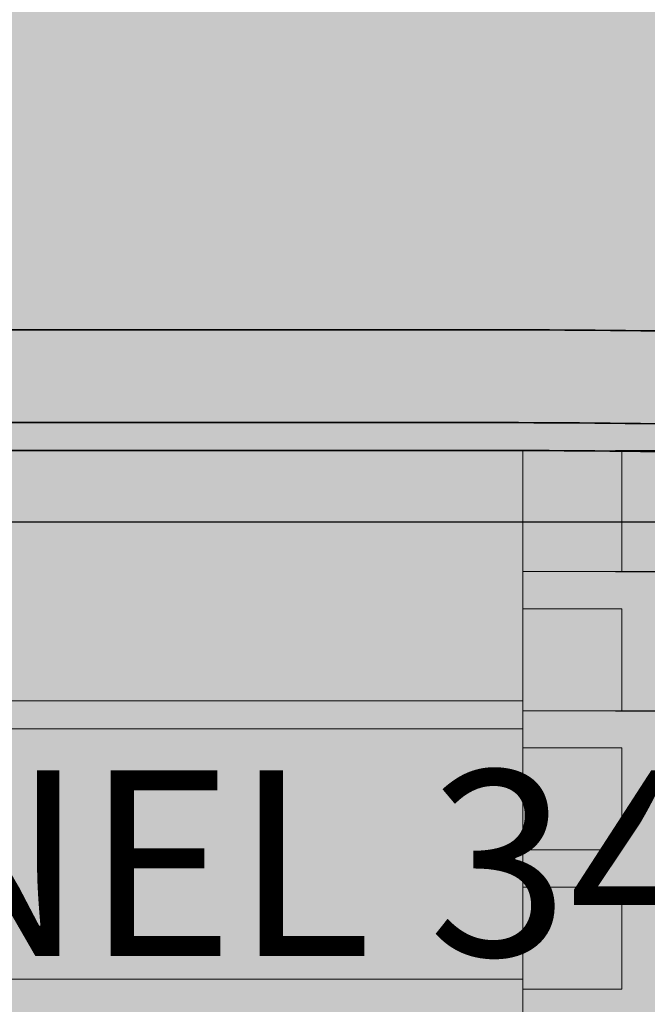
# Model space of a CAD drawing. Units: millimetres. Extents: x 130 to 1021, y 147 to 699.
# Tile 14 of 40: x 579 to 646, y 334 to 440. Entities that reach past the tile are written whole.
import ezdxf

# ---------------------------------------------------------------- set-up
doc = ezdxf.new("R2010")
doc.units = ezdxf.units.MM
doc.header["$MEASUREMENT"] = 0
for name, color, linetype, lineweight in [('A-ANNO-DIMS', 2, 'Continuous', 18), ('A-ELEV', 7, 'Continuous', 35), ('A-ELEV-PATT', 9, 'Continuous', 13), ('A-GLAZ', 4, 'Continuous', 18)]:
    doc.layers.add(name, color=color, linetype=linetype, lineweight=lineweight)
doc.styles.get("Standard").update_dxf_attribs({"font": 'arial.ttf'})
doc.dimstyles.get("Standard").update_dxf_attribs({"dimtxt": 20, "dimasz": 10, "dimexe": 10, "dimexo": 10, "dimgap": 5, "dimtad": 0, "dimtih": 1, "dimtoh": 1, "dimdec": 0, "dimzin": 0, "dimdsep": 46, "dimtxsty": 'Standard', "dimcen": 5, "dimadec": 0, "dimazin": 0, "dimtfac": 1, "dimtdec": 0, "dimtofl": 0, "dimtmove": 0, "dimatfit": 3, "dimfxl": 1, "dimtolj": 1, "dimtzin": 0, "dimarcsym": 0})

# ---------------------------------------------------------------- blocks, each defined once
blk = doc.blocks.new('*D7')
at = {"layer": 'A-ANNO-DIMS', "color": 0, "lineweight": -2, "transparency": 16777216}
for p, q in [((399.37, 349.45), (413.37, 349.45)), ((423.37, 349.45), (433.37, 349.45)), ((389.37, 344.55), (389.37, 339.45)), ((423.37, 344.55), (423.37, 339.45))]:
    blk.add_line(p, q, dxfattribs=at)
at = {"layer": 'A-ANNO-DIMS', "color": 0, "transparency": 16777216}
for points in [[(399.37, 351.11), (399.37, 347.78), (389.37, 349.45)], [(413.37, 351.11), (413.37, 347.78), (423.37, 349.45)]]:
    blk.add_solid(points, dxfattribs=at)
at = {"layer": 'Defpoints', "color": 0, "transparency": 16777216}
for p in [(389.37, 354.55), (423.37, 354.55), (423.37, 349.45)]:
    blk.add_point(p, dxfattribs=at)
at = {"layer": 'A-ANNO-DIMS', "color": 0, "transparency": 16777216, "insert": (582.04, 349.45), "char_height": 20, "attachment_point": 5}
blk.add_mtext('\\A1;DOOR PANEL 34 TYP.', dxfattribs=at)
blk = doc.blocks.new('*D11')
at = {"layer": 'A-ANNO-DIMS', "color": 0, "lineweight": -2, "transparency": 16777216}
for p, q in [((737.37, 648.7), (737.37, 149.74)), ((299.37, 566.95), (299.37, 149.74)), ((309.37, 159.74), (490.86, 159.74)), ((727.37, 159.74), (545.89, 159.74))]:
    blk.add_line(p, q, dxfattribs=at)
at = {"layer": 'A-ANNO-DIMS', "color": 0, "transparency": 16777216}
for points in [[(309.37, 161.41), (309.37, 158.07), (299.37, 159.74)], [(727.37, 161.41), (727.37, 158.07), (737.37, 159.74)]]:
    blk.add_solid(points, dxfattribs=at)
at = {"layer": 'Defpoints', "color": 0, "transparency": 16777216}
for p in [(737.37, 658.7), (299.37, 576.95), (737.37, 159.74)]:
    blk.add_point(p, dxfattribs=at)
at = {"layer": 'A-ANNO-DIMS', "color": 0, "transparency": 16777216, "insert": (518.37, 159.74), "char_height": 20, "attachment_point": 5}
blk.add_mtext('\\A1;438', dxfattribs=at)
blk = doc.blocks.new('*D24')
at = {"layer": 'A-ANNO-DIMS', "color": 0, "lineweight": -2, "transparency": 16777216}
for p, q in [((475.99, 209.04), (475.99, 696.25)), ((487.37, 671.95), (487.37, 696.25)), ((465.99, 686.25), (455.99, 686.25)), ((497.37, 686.25), (507.37, 686.25))]:
    blk.add_line(p, q, dxfattribs=at)
at = {"layer": 'A-ANNO-DIMS', "color": 0, "transparency": 16777216}
for points in [[(465.99, 687.91), (465.99, 684.58), (475.99, 686.25)], [(497.37, 687.91), (497.37, 684.58), (487.37, 686.25)]]:
    blk.add_solid(points, dxfattribs=at)
at = {"layer": 'Defpoints', "color": 0, "transparency": 16777216}
for p in [(487.37, 686.25), (487.37, 661.95), (475.99, 199.04)]:
    blk.add_point(p, dxfattribs=at)
at = {"layer": 'A-ANNO-DIMS', "color": 0, "transparency": 16777216, "insert": (553.02, 686.25), "char_height": 20, "attachment_point": 5}
blk.add_mtext('\\A1;11.385', dxfattribs=at)
blk = doc.blocks.new('*D27')
at = {"layer": 'A-ANNO-DIMS', "color": 0, "lineweight": -2, "transparency": 16777216}
for p, q in [((502.37, 593.95), (502.37, 696.25)), ((544.64, 396.26), (544.64, 696.25)), ((512.37, 686.25), (534.64, 686.25)), ((544.64, 686.25), (554.64, 686.25))]:
    blk.add_line(p, q, dxfattribs=at)
at = {"layer": 'A-ANNO-DIMS', "color": 0, "transparency": 16777216}
for points in [[(512.37, 687.91), (512.37, 684.58), (502.37, 686.25)], [(534.64, 687.91), (534.64, 684.58), (544.64, 686.25)]]:
    blk.add_solid(points, dxfattribs=at)
at = {"layer": 'Defpoints', "color": 0, "transparency": 16777216}
for p in [(544.64, 686.25), (502.37, 583.95), (544.64, 386.26)]:
    blk.add_point(p, dxfattribs=at)
at = {"layer": 'A-ANNO-DIMS', "color": 0, "transparency": 16777216, "insert": (593.78, 686.25), "char_height": 20, "attachment_point": 5}
blk.add_mtext('\\A1;42.26', dxfattribs=at)
blk = doc.blocks.new('*D28')
at = {"layer": 'A-ANNO-DIMS', "color": 0, "lineweight": -2, "transparency": 16777216}
for p, q in [((544.64, 396.26), (544.64, 696.25)), ((552.37, 593.95), (552.37, 696.25)), ((534.64, 686.25), (524.64, 686.25)), ((562.37, 686.25), (572.37, 686.25))]:
    blk.add_line(p, q, dxfattribs=at)
at = {"layer": 'A-ANNO-DIMS', "color": 0, "transparency": 16777216}
for points in [[(534.64, 687.91), (534.64, 684.58), (544.64, 686.25)], [(562.37, 687.91), (562.37, 684.58), (552.37, 686.25)]]:
    blk.add_solid(points, dxfattribs=at)
at = {"layer": 'Defpoints', "color": 0, "transparency": 16777216}
for p in [(552.37, 686.25), (552.37, 583.95), (544.64, 386.26)]:
    blk.add_point(p, dxfattribs=at)
at = {"layer": 'A-ANNO-DIMS', "color": 0, "transparency": 16777216, "insert": (611.06, 686.25), "char_height": 20, "attachment_point": 5}
blk.add_mtext('\\A1;7.738', dxfattribs=at)
blk = doc.blocks.new('*D51')
at = {"layer": 'A-ANNO-DIMS', "color": 0, "lineweight": -2, "transparency": 16777216}
for p, q in [((554.64, 386.26), (771.67, 386.26)), ((761.67, 376.26), (761.67, 348.67)), ((761.67, 290.66), (761.67, 318.25)), ((554.64, 280.66), (771.67, 280.66))]:
    blk.add_line(p, q, dxfattribs=at)
at = {"layer": 'A-ANNO-DIMS', "color": 0, "transparency": 16777216}
for points in [[(760.01, 376.26), (763.34, 376.26), (761.67, 386.26)], [(760.01, 290.66), (763.34, 290.66), (761.67, 280.66)]]:
    blk.add_solid(points, dxfattribs=at)
at = {"layer": 'Defpoints', "color": 0, "transparency": 16777216}
for p in [(544.64, 386.26), (761.67, 386.26), (544.64, 280.66)]:
    blk.add_point(p, dxfattribs=at)
at = {"layer": 'A-ANNO-DIMS', "color": 0, "transparency": 16777216, "insert": (761.67, 333.46), "char_height": 20, "attachment_point": 5}
blk.add_mtext('\\A1;105.6', dxfattribs=at)
blk = doc.blocks.new('*D52')
at = {"layer": 'A-ANNO-DIMS', "color": 0, "lineweight": -2, "transparency": 16777216}
for p, q in [((761.67, 403.95), (761.67, 413.95)), ((761.67, 413.95), (771.67, 413.95)), ((642.82, 393.95), (771.67, 393.95)), ((554.64, 386.26), (771.67, 386.26)), ((761.67, 376.26), (761.67, 366.26))]:
    blk.add_line(p, q, dxfattribs=at)
at = {"layer": 'A-ANNO-DIMS', "color": 0, "transparency": 16777216}
for points in [[(760.01, 403.95), (763.34, 403.95), (761.67, 393.95)], [(760.01, 376.26), (763.34, 376.26), (761.67, 386.26)]]:
    blk.add_solid(points, dxfattribs=at)
at = {"layer": 'Defpoints', "color": 0, "transparency": 16777216}
for p in [(632.82, 393.95), (761.67, 393.95), (544.64, 386.26)]:
    blk.add_point(p, dxfattribs=at)
at = {"layer": 'A-ANNO-DIMS', "color": 0, "transparency": 16777216, "insert": (810.34, 413.95), "char_height": 20, "attachment_point": 5}
blk.add_mtext('\\A1;7.683', dxfattribs=at)
blk = doc.blocks.new('*D53')
at = {"layer": 'A-ANNO-DIMS', "color": 0, "lineweight": -2, "transparency": 16777216}
for p, q in [((761.67, 413.69), (761.67, 423.69)), ((761.67, 423.69), (771.67, 423.69)), ((747.37, 403.69), (771.67, 403.69)), ((642.82, 393.95), (771.67, 393.95)), ((761.67, 383.95), (761.67, 373.95))]:
    blk.add_line(p, q, dxfattribs=at)
at = {"layer": 'A-ANNO-DIMS', "color": 0, "transparency": 16777216}
for points in [[(760.01, 413.69), (763.34, 413.69), (761.67, 403.69)], [(760.01, 383.95), (763.34, 383.95), (761.67, 393.95)]]:
    blk.add_solid(points, dxfattribs=at)
at = {"layer": 'Defpoints', "color": 0, "transparency": 16777216}
for p in [(737.37, 403.69), (761.67, 403.69), (632.82, 393.95)]:
    blk.add_point(p, dxfattribs=at)
at = {"layer": 'A-ANNO-DIMS', "color": 0, "transparency": 16777216, "insert": (810.42, 423.69), "char_height": 20, "attachment_point": 5}
blk.add_mtext('\\A1;9.743', dxfattribs=at)
blk = doc.blocks.new('*D54')
at = {"layer": 'A-ANNO-DIMS', "color": 0, "lineweight": -2, "transparency": 16777216}
for p, q in [((761.67, 473.95), (761.67, 483.95)), ((497.37, 463.95), (771.67, 463.95)), ((747.37, 403.69), (771.67, 403.69)), ((761.67, 393.69), (761.67, 383.69))]:
    blk.add_line(p, q, dxfattribs=at)
at = {"layer": 'A-ANNO-DIMS', "color": 0, "transparency": 16777216}
for points in [[(760.01, 473.95), (763.34, 473.95), (761.67, 463.95)], [(760.01, 393.69), (763.34, 393.69), (761.67, 403.69)]]:
    blk.add_solid(points, dxfattribs=at)
at = {"layer": 'Defpoints', "color": 0, "transparency": 16777216}
for p in [(487.37, 463.95), (761.67, 463.95), (737.37, 403.69)]:
    blk.add_point(p, dxfattribs=at)
at = {"layer": 'A-ANNO-DIMS', "color": 0, "transparency": 16777216, "insert": (761.67, 433.82), "char_height": 20, "attachment_point": 5}
blk.add_mtext('\\A1;60.26', dxfattribs=at)
blk = doc.blocks.new('*D61')
at = {"layer": 'A-ANNO-DIMS', "color": 0, "lineweight": -2, "transparency": 16777216}
for p, q in [((761.67, 390.89), (761.67, 400.89)), ((642.82, 380.89), (771.67, 380.89)), ((642.82, 365.89), (771.67, 365.89)), ((761.67, 355.89), (761.67, 345.89)), ((761.67, 345.89), (751.67, 345.89))]:
    blk.add_line(p, q, dxfattribs=at)
at = {"layer": 'A-ANNO-DIMS', "color": 0, "transparency": 16777216}
for points in [[(760.01, 390.89), (763.34, 390.89), (761.67, 380.89)], [(760.01, 355.89), (763.34, 355.89), (761.67, 365.89)]]:
    blk.add_solid(points, dxfattribs=at)
at = {"layer": 'Defpoints', "color": 0, "transparency": 16777216}
for p in [(632.82, 380.89), (632.82, 365.89), (761.67, 365.89)]:
    blk.add_point(p, dxfattribs=at)
at = {"layer": 'A-ANNO-DIMS', "color": 0, "transparency": 16777216, "insert": (733.22, 345.89), "char_height": 20, "attachment_point": 5}
blk.add_mtext('\\A1;15', dxfattribs=at)
blk = doc.blocks.new('*D65')
at = {"layer": 'A-ANNO-DIMS', "color": 0, "lineweight": -2, "transparency": 16777216}
for p, q in [((495.46, 509.13), (472.51, 423.11)), ((505.46, 509.13), (495.46, 509.13)), ((427.37, 248.98), (427.37, 258.98)), ((422.37, 253.98), (432.37, 253.98))]:
    blk.add_line(p, q, dxfattribs=at)
at = {"layer": 'A-ANNO-DIMS', "color": 0, "transparency": 16777216}
blk.add_solid([(470.9, 423.54), (474.12, 422.68), (469.93, 413.45)], dxfattribs=at)
at = {"layer": 'Defpoints', "color": 0, "transparency": 16777216}
for p in [(469.93, 413.45), (427.37, 253.98)]:
    blk.add_point(p, dxfattribs=at)
at = {"layer": 'A-ANNO-DIMS', "color": 0, "transparency": 16777216, "insert": (561.62, 509.13), "char_height": 20, "attachment_point": 5}
blk.add_mtext('\\A1;R165.05', dxfattribs=at)
blk = doc.blocks.new('*D67')
at = {"layer": 'A-ANNO-DIMS', "color": 0, "lineweight": -2, "transparency": 16777216}
for p, q in [((479.76, 492.43), (462.14, 412.22)), ((489.76, 492.43), (479.76, 492.43)), ((427.07, 247.5), (427.07, 257.5)), ((422.07, 252.5), (432.07, 252.5))]:
    blk.add_line(p, q, dxfattribs=at)
at = {"layer": 'A-ANNO-DIMS', "color": 0, "transparency": 16777216}
blk.add_solid([(460.52, 412.58), (463.77, 411.87), (460, 402.46)], dxfattribs=at)
at = {"layer": 'Defpoints', "color": 0, "transparency": 16777216}
for p in [(460, 402.46), (427.07, 252.5)]:
    blk.add_point(p, dxfattribs=at)
at = {"layer": 'A-ANNO-DIMS', "color": 0, "transparency": 16777216, "insert": (545.84, 492.43), "char_height": 20, "attachment_point": 5}
blk.add_mtext('\\A1;R153.53', dxfattribs=at)
blk = doc.blocks.new('*D69')
at = {"layer": 'A-ANNO-DIMS', "color": 0, "lineweight": -2, "transparency": 16777216}
for p, q in [((507.75, 572.26), (483.09, 501.81)), ((517.75, 572.26), (507.75, 572.26)), ((433.19, 354.23), (433.19, 364.23)), ((428.19, 359.23), (438.19, 359.23))]:
    blk.add_line(p, q, dxfattribs=at)
at = {"layer": 'A-ANNO-DIMS', "color": 0, "transparency": 16777216}
blk.add_solid([(481.52, 502.36), (484.66, 501.26), (479.79, 492.37)], dxfattribs=at)
at = {"layer": 'Defpoints', "color": 0, "transparency": 16777216}
for p in [(479.79, 492.37), (433.19, 359.23)]:
    blk.add_point(p, dxfattribs=at)
at = {"layer": 'A-ANNO-DIMS', "color": 0, "transparency": 16777216, "insert": (573.82, 572.26), "char_height": 20, "attachment_point": 5}
blk.add_mtext('\\A1;R141.06', dxfattribs=at)
blk = doc.blocks.new('*D71')
at = {"layer": 'A-ANNO-DIMS', "color": 0, "lineweight": -2, "transparency": 16777216}
for p, q in [((492.11, 581.61), (472.54, 512.67)), ((502.11, 581.61), (492.11, 581.61)), ((432.65, 367.11), (432.65, 377.11)), ((427.65, 372.11), (437.65, 372.11))]:
    blk.add_line(p, q, dxfattribs=at)
at = {"layer": 'A-ANNO-DIMS', "color": 0, "transparency": 16777216}
blk.add_solid([(470.94, 513.12), (474.15, 512.21), (469.81, 503.05)], dxfattribs=at)
at = {"layer": 'Defpoints', "color": 0, "transparency": 16777216}
for p in [(469.81, 503.05), (432.65, 372.11)]:
    blk.add_point(p, dxfattribs=at)
at = {"layer": 'A-ANNO-DIMS', "color": 0, "transparency": 16777216, "insert": (548.49, 581.61), "char_height": 20, "attachment_point": 5}
blk.add_mtext('\\A1;R136.1', dxfattribs=at)

msp = doc.modelspace()

# ---------------------------------------------------------------- hatches: boundary and pattern name
at = {"layer": 'A-ELEV-PATT'}
h = msp.add_hatch(color=256, dxfattribs=at)
h.dxf.hatch_style = 1
h.paths.add_polyline_path([(737.3738, 658.6988, 0.01359606), (632.4019, 661.9473), (607.3738, 661.9473), (487.3738, 661.9473), (487.3738, 649.9473), (607.3738, 649.9473), (632.3794, 649.9473, -0.01368411), (737.3738, 646.6784)])
h.paths.add_polyline_path([(732.3738, 643.9599, 0.01305286), (632.3738, 646.9473), (607.3738, 646.9473), (487.3738, 646.9473), (487.3738, 596.9473), (632.3738, 596.9473, -0.01305286), (732.3738, 593.9599)])
h.paths.add_polyline_path([(737.3738, 593.6732, 0.01370629), (632.3738, 596.9473), (487.3738, 596.9473), (487.3738, 586.9473), (632.355, 586.9473, -0.01378075), (737.3738, 583.6559)])
h.paths.add_polyline_path([(447.3738, 646.9473), (307.3738, 646.9473), (302.3738, 646.9473), (302.3738, 634.9473), (447.3738, 634.9473)])
h.paths.add_polyline_path([(447.3738, 631.9473), (307.3738, 631.9473), (307.3738, 586.9473), (447.3738, 586.9473)])
h.paths.add_polyline_path([(447.3738, 586.9473), (307.3738, 586.9473), (302.3738, 586.9473), (302.3738, 576.9473), (447.3738, 576.9473)])
h.paths.add_polyline_path([(447.3738, 573.9473), (367.3738, 573.9473), (367.3738, 539.9473), (447.3738, 539.9473)])
h.paths.add_polyline_path([(447.3738, 537.9473), (367.3738, 537.9473), (367.3738, 507.9473), (400.392, 507.4253, -0.00172798), (401.3281, 507.6451, -0.52200255), (425.6117, 511.0391, -0.03918489), (447.3738, 510.4359), (447.3738, 510.7883)])
h.paths.add_polyline_path([(394.7238, 505.9473), (367.3738, 505.9473), (367.3738, 476.9473, -0.0146512), (375.8501, 480.2159), (376.1506, 499.2266, -0.03554194)])
h.paths.add_polyline_path([(632.3738, 583.9473), (552.3738, 583.9473), (552.3738, 550.9473), (632.3738, 550.9473)])
h.paths.add_polyline_path([(632.3738, 548.9473), (552.3738, 548.9473), (552.3738, 515.9473), (632.3738, 515.9473)])
h.paths.add_polyline_path([(632.3738, 513.9473), (552.3738, 513.9473), (552.3738, 476.9473), (632.3738, 476.9473)])
h.paths.add_polyline_path([(737.3738, 473.6903, 0.01363261), (632.3926, 476.9473), (552.3738, 476.9473), (487.3738, 476.9473), (487.3738, 466.9473), (632.3738, 466.9473, -0.01370629), (737.3738, 463.6732)])
h.paths.add_polyline_path([(732.3738, 460.9552, 0.01307409), (632.3681, 463.9473), (487.3738, 463.9473), (487.3738, 407.735, -0.00322862), (489.3544, 406.9473), (632.3926, 406.9473, -0.01298259), (732.3738, 403.9755)])
h.paths.add_polyline_path([(487.3738, 463.9473, 0.20132998), (367.3738, 463.9473), (367.3738, 407.735, -0.18820307), (487.3738, 407.735)])
h.paths.add_polyline_path([(367.3738, 476.9473), (367.3738, 466.9473, -0.20133085), (487.3738, 466.9473), (487.3738, 476.9473, 0.20132998)])
h.paths.add_polyline_path([(367.3738, 463.9473), (307.3738, 463.9473), (307.3738, 401.9473), (357.9413, 401.9473), (367.3738, 407.735)])
h.paths.add_polyline_path([(367.3738, 476.9473), (302.3738, 476.9473), (302.3738, 466.9473), (367.3738, 466.9473)])
h.paths.add_polyline_path([(632.8184, 366.9453), (552.3738, 366.9453), (552.3738, 393.9473), (632.8184, 393.9473)])
h.paths.add_polyline_path([(632.8184, 357.2114), (632.8184, 363.9453), (552.3738, 363.9453), (552.3738, 357.2114), (552.3738, 336.9453), (632.8184, 336.9453)])
h.paths.add_polyline_path([(632.8184, 333.9453), (552.3738, 333.9453), (552.3738, 306.9453), (632.8184, 306.9453)])
h.paths.add_polyline_path([(632.8184, 303.9453), (552.3738, 303.9453), (552.3738, 273.9473), (632.355, 273.9473, 0.00006077), (632.8184, 273.9491)])
h.paths.add_polyline_path([(737.3738, 403.6903, 0.01363261), (632.3926, 406.9473), (489.3544, 406.9473, 0.19154808), (367.3738, 407.735), (367.3738, 396.9473, -0.20133085), (487.3738, 396.9473), (632.3738, 396.9473, -0.01370629), (737.3738, 393.6732)])
h.paths.add_polyline_path([(357.9413, 401.9473), (307.3738, 401.9473), (307.3738, 391.9473), (357.9413, 391.9473)])
h.paths.add_polyline_path([(357.9413, 357.2114), (357.9413, 388.9473), (307.3738, 388.9473), (307.3738, 357.2114), (307.3738, 273.9473), (357.9413, 273.9473)])
h.paths.add_polyline_path([(732.3738, 263.93, -0.0130317), (632.3794, 260.9473), (466.7667, 260.9473), (466.7667, 240.9473), (469.8406, 236.978), (469.8406, 221.978), (472.9145, 218.0087), (472.9145, 213.9473), (607.3738, 213.9473), (732.3738, 213.9473)])
h.paths.add_polyline_path([(732.3738, 290.889), (722.479, 290.889), (722.479, 301.889), (732.3738, 301.889), (732.3738, 305.889), (722.479, 305.889), (722.479, 316.889), (732.3738, 316.889), (732.3738, 320.889), (722.479, 320.889), (722.479, 331.889), (732.3738, 331.889), (732.3738, 335.889), (722.479, 335.889), (722.479, 346.889), (732.3738, 346.889), (732.3738, 350.889), (722.479, 350.889), (722.479, 361.889), (732.3738, 361.889), (732.3738, 365.889), (722.479, 365.889), (722.479, 376.889), (732.3738, 376.889), (732.3738, 380.889), (722.479, 380.889), (722.479, 391.4848, 0.00052326), (718.479, 391.6843), (718.479, 380.889), (707.479, 380.889), (707.479, 392.1896, 0.00052307), (703.479, 392.3576), (703.479, 380.889), (692.479, 380.889), (692.479, 392.7765, 0.00052292), (688.479, 392.9131), (688.479, 380.889), (677.479, 380.889), (677.479, 393.2456, 0.00052279), (673.479, 393.3508), (673.479, 380.889), (662.479, 380.889), (662.479, 393.597, 0.0005227), (658.479, 393.6709), (658.479, 380.889), (647.479, 380.889), (647.479, 393.8308, 0.00052264), (643.479, 393.8732), (643.479, 380.889), (632.8184, 380.889), (632.8184, 376.889), (643.479, 376.889), (643.479, 365.889), (632.8184, 365.889), (632.8184, 361.889), (643.479, 361.889), (643.479, 350.889), (632.8184, 350.889), (632.8184, 346.889), (643.479, 346.889), (643.479, 335.889), (632.8184, 335.889), (632.8184, 331.889), (643.479, 331.889), (643.479, 320.889), (632.8184, 320.889), (632.8184, 316.889), (643.479, 316.889), (643.479, 305.889), (632.8184, 305.889), (632.8184, 301.889), (643.479, 301.889), (643.479, 290.889), (632.8184, 290.889), (632.8184, 286.889), (643.479, 286.889), (643.479, 274.0217, 0.00052456), (647.479, 274.0643), (647.479, 286.889), (658.479, 286.889), (658.479, 274.2248, 0.00052462), (662.479, 274.2989), (662.479, 286.889), (673.479, 286.889), (673.479, 274.546, 0.00052471), (677.479, 274.6516), (677.479, 286.889), (688.479, 286.889), (688.479, 274.9853, 0.00052484), (692.479, 275.1224), (692.479, 286.889), (703.479, 286.889), (703.479, 275.5429, 0.000525), (707.479, 275.7115), (707.479, 286.889), (718.479, 286.889), (718.479, 276.2187, 0.00052519), (722.479, 276.4189), (722.479, 286.889), (732.3738, 286.889)])
h.paths.add_polyline_path([(718.479, 290.889), (707.479, 290.889), (707.479, 301.889), (718.479, 301.889)], flags=16)
h.paths.add_polyline_path([(703.479, 290.889), (692.479, 290.889), (692.479, 301.889), (703.479, 301.889)], flags=16)
h.paths.add_polyline_path([(718.479, 305.889), (707.479, 305.889), (707.479, 316.889), (718.479, 316.889)], flags=16)
h.paths.add_polyline_path([(703.479, 305.889), (692.479, 305.889), (692.479, 316.889), (703.479, 316.889)], flags=16)
h.paths.add_polyline_path([(688.479, 290.889), (677.479, 290.889), (677.479, 301.889), (688.479, 301.889)], flags=16)
h.paths.add_polyline_path([(718.479, 320.889), (707.479, 320.889), (707.479, 331.889), (718.479, 331.889)], flags=16)
h.paths.add_polyline_path([(688.479, 305.889), (677.479, 305.889), (677.479, 316.889), (688.479, 316.889)], flags=16)
h.paths.add_polyline_path([(703.479, 320.889), (692.479, 320.889), (692.479, 331.889), (703.479, 331.889)], flags=16)
h.paths.add_polyline_path([(688.479, 320.889), (677.479, 320.889), (677.479, 331.889), (688.479, 331.889)], flags=16)
h.paths.add_polyline_path([(673.479, 290.889), (662.479, 290.889), (662.479, 301.889), (673.479, 301.889)], flags=16)
h.paths.add_polyline_path([(718.479, 335.889), (707.479, 335.889), (707.479, 346.889), (718.479, 346.889)], flags=16)
h.paths.add_polyline_path([(673.479, 305.889), (662.479, 305.889), (662.479, 316.889), (673.479, 316.889)], flags=16)
h.paths.add_polyline_path([(703.479, 335.889), (692.479, 335.889), (692.479, 346.889), (703.479, 346.889)], flags=16)
h.paths.add_polyline_path([(673.479, 320.889), (662.479, 320.889), (662.479, 331.889), (673.479, 331.889)], flags=16)
h.paths.add_polyline_path([(688.479, 335.889), (677.479, 335.889), (677.479, 346.889), (688.479, 346.889)], flags=16)
h.paths.add_polyline_path([(658.479, 290.889), (647.479, 290.889), (647.479, 301.889), (658.479, 301.889)], flags=16)
h.paths.add_polyline_path([(718.479, 350.889), (707.479, 350.889), (707.479, 361.889), (718.479, 361.889)], flags=16)
h.paths.add_polyline_path([(658.479, 305.889), (647.479, 305.889), (647.479, 316.889), (658.479, 316.889)], flags=16)
h.paths.add_polyline_path([(703.479, 350.889), (692.479, 350.889), (692.479, 361.889), (703.479, 361.889)], flags=16)
h.paths.add_polyline_path([(673.479, 335.889), (662.479, 335.889), (662.479, 346.889), (673.479, 346.889)], flags=16)
h.paths.add_polyline_path([(658.479, 320.889), (647.479, 320.889), (647.479, 331.889), (658.479, 331.889)], flags=16)
h.paths.add_polyline_path([(688.479, 350.889), (677.479, 350.889), (677.479, 361.889), (688.479, 361.889)], flags=16)
h.paths.add_polyline_path([(718.479, 365.889), (707.479, 365.889), (707.479, 376.889), (718.479, 376.889)], flags=16)
h.paths.add_polyline_path([(658.479, 335.889), (647.479, 335.889), (647.479, 346.889), (658.479, 346.889)], flags=16)
h.paths.add_polyline_path([(673.479, 350.889), (662.479, 350.889), (662.479, 361.889), (673.479, 361.889)], flags=16)
h.paths.add_polyline_path([(703.479, 365.889), (692.479, 365.889), (692.479, 376.889), (703.479, 376.889)], flags=16)
h.paths.add_polyline_path([(688.479, 365.889), (677.479, 365.889), (677.479, 376.889), (688.479, 376.889)], flags=16)
h.paths.add_polyline_path([(658.479, 350.889), (647.479, 350.889), (647.479, 361.889), (658.479, 361.889)], flags=16)
h.paths.add_polyline_path([(673.479, 365.889), (662.479, 365.889), (662.479, 376.889), (673.479, 376.889)], flags=16)
h.paths.add_polyline_path([(658.479, 365.889), (647.479, 365.889), (647.479, 376.889), (658.479, 376.889)], flags=16)
h.paths.add_polyline_path([(732.3738, 503.9786), (722.3392, 503.9786), (722.3392, 514.9786), (732.3738, 514.9786), (732.3738, 518.9786), (722.3392, 518.9786), (722.3392, 529.9786), (732.3738, 529.9786), (732.3738, 533.9786), (722.3392, 533.9786), (722.3392, 544.9786), (732.3738, 544.9786), (732.3738, 546.9473), (732.3738, 548.9786), (722.3392, 548.9786), (722.3392, 559.9786), (732.3738, 559.9786), (732.3738, 563.9786), (722.3392, 563.9786), (722.3392, 574.9786), (732.3738, 574.9786), (732.3738, 578.9786), (722.3392, 578.9786), (722.3392, 581.4789, 0.00052601), (718.3392, 581.6791), (718.3392, 578.9786), (707.3392, 578.9786), (707.3392, 582.1863, 0.00052582), (703.3392, 582.355), (703.3392, 578.9786), (692.3392, 578.9786), (692.3392, 582.7752, 0.00052566), (688.3392, 582.9123), (688.3392, 578.9786), (677.3392, 578.9786), (677.3392, 583.2457, 0.00052554), (673.3392, 583.3512), (673.3392, 578.9786), (662.3392, 578.9786), (662.3392, 583.5978, 0.00052545), (658.3392, 583.6718), (658.3392, 578.9786), (647.3392, 578.9786), (647.3392, 583.8317, 0.00052539), (643.3392, 583.8741), (643.3392, 578.9786), (632.3738, 578.9786), (632.3738, 574.9786), (643.3392, 574.9786), (643.3392, 563.9786), (632.3738, 563.9786), (632.3738, 559.9786), (643.3392, 559.9786), (643.3392, 548.9786), (632.3738, 548.9786), (632.3738, 544.9786), (643.3392, 544.9786), (643.3392, 533.9786), (632.3738, 533.9786), (632.3738, 529.9786), (643.3392, 529.9786), (643.3392, 518.9786), (632.3738, 518.9786), (632.3738, 515.9473), (632.3738, 514.9786), (643.3392, 514.9786), (643.3392, 503.9786), (632.3738, 503.9786), (632.3738, 499.9786), (643.3392, 499.9786), (643.3392, 488.9786), (632.3738, 488.9786), (632.3738, 484.9786), (643.3392, 484.9786), (643.3392, 476.8751, -0.00051911), (647.3392, 476.8332), (647.3392, 484.9786), (658.3392, 484.9786), (658.3392, 476.6752, -0.00051917), (662.3392, 476.6022), (662.3392, 484.9786), (673.3392, 484.9786), (673.3392, 476.3585, -0.00051926), (677.3392, 476.2543), (677.3392, 484.9786), (688.3392, 484.9786), (688.3392, 475.9248, -0.00051938), (692.3392, 475.7894), (692.3392, 484.9786), (703.3392, 484.9786), (703.3392, 475.3741, -0.00051953), (707.3392, 475.2075), (707.3392, 484.9786), (718.3392, 484.9786), (718.3392, 474.7064, -0.00051972), (722.3392, 474.5086), (722.3392, 484.9786), (732.3738, 484.9786), (732.3738, 488.9786), (722.3392, 488.9786), (722.3392, 499.9786), (732.3738, 499.9786)])
h.paths.add_polyline_path([(718.3392, 503.9786), (707.3392, 503.9786), (707.3392, 514.9786), (718.3392, 514.9786)], flags=16)
h.paths.add_polyline_path([(718.3392, 499.9786), (718.3392, 488.9786), (707.3392, 488.9786), (707.3392, 499.9786)], flags=16)
h.paths.add_polyline_path([(718.3392, 518.9786), (707.3392, 518.9786), (707.3392, 529.9786), (718.3392, 529.9786)], flags=16)
h.paths.add_polyline_path([(703.3392, 503.9786), (692.3392, 503.9786), (692.3392, 514.9786), (703.3392, 514.9786)], flags=16)
h.paths.add_polyline_path([(703.3392, 499.9786), (703.3392, 488.9786), (692.3392, 488.9786), (692.3392, 499.9786)], flags=16)
h.paths.add_polyline_path([(703.3392, 518.9786), (692.3392, 518.9786), (692.3392, 529.9786), (703.3392, 529.9786)], flags=16)
h.paths.add_polyline_path([(718.3392, 533.9786), (707.3392, 533.9786), (707.3392, 544.9786), (718.3392, 544.9786)], flags=16)
h.paths.add_polyline_path([(688.3392, 503.9786), (677.3392, 503.9786), (677.3392, 514.9786), (688.3392, 514.9786)], flags=16)
h.paths.add_polyline_path([(688.3392, 499.9786), (688.3392, 488.9786), (677.3392, 488.9786), (677.3392, 499.9786)], flags=16)
h.paths.add_polyline_path([(703.3392, 533.9786), (692.3392, 533.9786), (692.3392, 544.9786), (703.3392, 544.9786)], flags=16)
h.paths.add_polyline_path([(688.3392, 518.9786), (677.3392, 518.9786), (677.3392, 529.9786), (688.3392, 529.9786)], flags=16)
h.paths.add_polyline_path([(688.3392, 533.9786), (677.3392, 533.9786), (677.3392, 544.9786), (688.3392, 544.9786)], flags=16)
h.paths.add_polyline_path([(718.3392, 548.9786), (707.3392, 548.9786), (707.3392, 559.9786), (718.3392, 559.9786)], flags=16)
h.paths.add_polyline_path([(673.3392, 503.9786), (662.3392, 503.9786), (662.3392, 514.9786), (673.3392, 514.9786)], flags=16)
h.paths.add_polyline_path([(673.3392, 499.9786), (673.3392, 488.9786), (662.3392, 488.9786), (662.3392, 499.9786)], flags=16)
h.paths.add_polyline_path([(703.3392, 548.9786), (692.3392, 548.9786), (692.3392, 559.9786), (703.3392, 559.9786)], flags=16)
h.paths.add_polyline_path([(673.3392, 518.9786), (662.3392, 518.9786), (662.3392, 529.9786), (673.3392, 529.9786)], flags=16)
h.paths.add_polyline_path([(688.3392, 548.9786), (677.3392, 548.9786), (677.3392, 559.9786), (688.3392, 559.9786)], flags=16)
h.paths.add_polyline_path([(673.3392, 533.9786), (662.3392, 533.9786), (662.3392, 544.9786), (673.3392, 544.9786)], flags=16)
h.paths.add_polyline_path([(718.3392, 563.9786), (707.3392, 563.9786), (707.3392, 574.9786), (718.3392, 574.9786)], flags=16)
h.paths.add_polyline_path([(658.3392, 503.9786), (647.3392, 503.9786), (647.3392, 514.9786), (658.3392, 514.9786)], flags=16)
h.paths.add_polyline_path([(658.3392, 499.9786), (658.3392, 488.9786), (647.3392, 488.9786), (647.3392, 499.9786)], flags=16)
h.paths.add_polyline_path([(703.3392, 563.9786), (692.3392, 563.9786), (692.3392, 574.9786), (703.3392, 574.9786)], flags=16)
h.paths.add_polyline_path([(658.3392, 518.9786), (647.3392, 518.9786), (647.3392, 529.9786), (658.3392, 529.9786)], flags=16)
h.paths.add_polyline_path([(673.3392, 548.9786), (662.3392, 548.9786), (662.3392, 559.9786), (673.3392, 559.9786)], flags=16)
h.paths.add_polyline_path([(688.3392, 563.9786), (677.3392, 563.9786), (677.3392, 574.9786), (688.3392, 574.9786)], flags=16)
h.paths.add_polyline_path([(658.3392, 533.9786), (647.3392, 533.9786), (647.3392, 544.9786), (658.3392, 544.9786)], flags=16)
h.paths.add_polyline_path([(673.3392, 563.9786), (662.3392, 563.9786), (662.3392, 574.9786), (673.3392, 574.9786)], flags=16)
h.paths.add_polyline_path([(658.3392, 548.9786), (647.3392, 548.9786), (647.3392, 559.9786), (658.3392, 559.9786)], flags=16)
h.paths.add_polyline_path([(658.3392, 563.9786), (647.3392, 563.9786), (647.3392, 574.9786), (658.3392, 574.9786)], flags=16)
h = msp.add_hatch(color=256, dxfattribs=at)
h.dxf.hatch_style = 1
h.paths.add_polyline_path([(447.3738, 576.9473), (302.3738, 576.9473), (302.3738, 573.9473), (447.3738, 573.9473)])
h.paths.add_polyline_path([(487.3738, 583.9473), (487.3738, 586.9473), (447.3738, 576.9473), (447.3738, 573.9473)])
h.paths.add_polyline_path([(632.355, 586.9473), (487.3738, 586.9473), (487.3738, 583.9473), (632.3738, 583.9473), (632.3738, 583.9472, -0.01380003), (737.3738, 580.6507), (737.3738, 583.6559, 0.01378075)])
h.paths.add_polyline_path([(367.3738, 466.9473), (302.3738, 466.9473), (302.3738, 463.9473), (367.3738, 463.9473)])
h.paths.add_polyline_path([(487.3738, 463.9473), (487.3738, 466.9473, 0.20133085), (367.3738, 466.9473), (367.3738, 463.9473, -0.20132998)])
h.paths.add_polyline_path([(632.3738, 466.9473), (487.3738, 466.9473), (487.3738, 463.9473), (632.3681, 463.9473, -0.01372855), (737.3738, 460.6681), (737.3738, 463.6732, 0.01370629)])
h.paths.add_polyline_path([(632.3738, 396.9473), (487.3738, 396.9473, 0.20133085), (367.3738, 396.9473), (367.3738, 393.9473, -0.20237172), (486.7667, 393.9473), (632.3681, 393.9473, -0.01372855), (737.3738, 390.6681), (737.3738, 393.6732, 0.01370629)])
h.paths.add_polyline_path([(357.9413, 391.9473), (307.3738, 391.9473), (307.3738, 388.9473), (357.9413, 388.9473)])
h.paths.add_polyline_path([(367.3738, 393.9473), (367.3738, 396.9473), (357.9413, 391.924), (357.9413, 388.9473), (358.058, 388.9473)])
h.paths.add_polyline_path([(737.3738, 264.2162), (737.3738, 267.2214, -0.01370629), (632.3738, 263.9473), (463.7667, 263.9473), (466.7667, 260.9473), (632.3794, 260.9473, 0.01368411)])
h.paths.add_polyline_path([(463.7667, 263.9473), (447.3738, 263.9473), (450.3738, 260.9473), (466.7667, 260.9473)])
h.paths.add_polyline_path([(447.3738, 263.9473), (432.3738, 263.9473), (432.3738, 260.9473), (450.3738, 260.9473)])
h.paths.add_polyline_path([(382.3738, 263.9473), (357.9413, 263.9473), (357.9413, 260.9473), (382.3738, 260.9473)])
h.paths.add_polyline_path([(357.9413, 263.9473), (307.3738, 263.9473), (307.3738, 260.9473), (357.9413, 260.9473)])
h = msp.add_hatch(color=256, dxfattribs=at)
h.dxf.hatch_style = 1
h.paths.add_polyline_path([(447.3738, 537.9473), (447.3738, 539.9473), (367.3738, 539.9473), (367.3738, 537.9473)])
h.paths.add_polyline_path([(394.7238, 505.9473, -0.0105284), (400.392, 507.4253), (367.3738, 507.9473), (367.3738, 505.9473)])
h.paths.add_polyline_path([(547.7773, 546.9473), (547.7773, 548.9473), (502.3738, 548.9473), (502.3738, 546.9473)])
h.paths.add_polyline_path([(632.3738, 548.9473), (632.3738, 550.9473), (552.3738, 550.9473), (552.3738, 548.9473)])
h.paths.add_polyline_path([(632.3738, 513.9473), (632.3738, 515.9473), (552.3738, 515.9473), (552.3738, 513.9473)])
h.paths.add_polyline_path([(544.6354, 360.9453), (544.6354, 363.9453), (486.7667, 363.9454), (486.7667, 360.9454)])
h.paths.add_polyline_path([(632.8184, 363.9453), (632.8184, 366.9453), (552.3738, 366.9453), (552.3738, 363.9453)])
h.paths.add_polyline_path([(632.8184, 333.9453), (632.8184, 336.9453), (552.3738, 336.9453), (552.3738, 333.9453)])
h.paths.add_polyline_path([(552.3738, 306.9453), (552.3738, 303.9453), (632.8184, 303.9453), (632.8184, 306.9453)])
h = msp.add_hatch(color=256, dxfattribs=at)
h.set_gradient(color1=(0, 153, 204), color2=(102, 204, 127))
h.paths.add_polyline_path([(643.479, 286.889), (632.8184, 286.889), (632.8184, 273.9491, 0.00139799), (643.479, 274.0217)])
h.paths.add_polyline_path([(647.479, 274.0643, 0.00144261), (658.479, 274.2248), (658.479, 286.889), (647.479, 286.889)])
h.paths.add_polyline_path([(662.479, 274.2989, 0.00144282), (673.479, 274.546), (673.479, 286.889), (662.479, 286.889)])
h.paths.add_polyline_path([(677.479, 274.6516, 0.00144312), (688.479, 274.9853), (688.479, 286.889), (677.479, 286.889)])
h.paths.add_polyline_path([(703.479, 275.5429), (703.479, 286.889), (692.479, 286.889), (692.479, 275.1224, 0.00144351)])
h.paths.add_polyline_path([(707.479, 275.7115, 0.00144399), (718.479, 276.2187), (718.479, 286.889), (707.479, 286.889)])
h.paths.add_polyline_path([(722.479, 276.4189, 0.0012994), (732.3738, 276.9505), (732.3738, 286.889), (722.479, 286.889)])
h.paths.add_polyline_path([(722.479, 290.889), (732.3738, 290.889), (732.3738, 301.889), (722.479, 301.889)])
h.paths.add_polyline_path([(718.479, 301.889), (707.479, 301.889), (707.479, 290.889), (718.479, 290.889)])
h.paths.add_polyline_path([(703.479, 301.889), (692.479, 301.889), (692.479, 290.889), (703.479, 290.889)])
h.paths.add_polyline_path([(677.479, 290.889), (688.479, 290.889), (688.479, 301.889), (677.479, 301.889)])
h.paths.add_polyline_path([(673.479, 301.889), (662.479, 301.889), (662.479, 290.889), (673.479, 290.889)])
h.paths.add_polyline_path([(658.479, 301.889), (647.479, 301.889), (647.479, 290.889), (658.479, 290.889)])
h.paths.add_polyline_path([(643.479, 301.889), (632.8184, 301.889), (632.8184, 290.889), (643.479, 290.889)])
h.paths.add_polyline_path([(643.479, 316.889), (632.8184, 316.889), (632.8184, 305.889), (643.479, 305.889)])
h.paths.add_polyline_path([(647.479, 305.889), (658.479, 305.889), (658.479, 316.889), (647.479, 316.889)])
h.paths.add_polyline_path([(662.479, 305.889), (673.479, 305.889), (673.479, 316.889), (662.479, 316.889)])
h.paths.add_polyline_path([(688.479, 316.889), (677.479, 316.889), (677.479, 305.889), (688.479, 305.889)])
h.paths.add_polyline_path([(692.479, 305.889), (703.479, 305.889), (703.479, 316.889), (692.479, 316.889)])
h.paths.add_polyline_path([(707.479, 305.889), (718.479, 305.889), (718.479, 316.889), (707.479, 316.889)])
h.paths.add_polyline_path([(722.479, 305.889), (732.3738, 305.889), (732.3738, 316.889), (722.479, 316.889)])
h.paths.add_polyline_path([(732.3738, 331.889), (722.479, 331.889), (722.479, 320.889), (732.3738, 320.889)])
h.paths.add_polyline_path([(718.479, 331.889), (707.479, 331.889), (707.479, 320.889), (718.479, 320.889)])
h.paths.add_polyline_path([(703.479, 331.889), (692.479, 331.889), (692.479, 320.889), (703.479, 320.889)])
h.paths.add_polyline_path([(688.479, 331.889), (677.479, 331.889), (677.479, 320.889), (688.479, 320.889)])
h.paths.add_polyline_path([(673.479, 331.889), (662.479, 331.889), (662.479, 320.889), (673.479, 320.889)])
h.paths.add_polyline_path([(647.479, 320.889), (658.479, 320.889), (658.479, 331.889), (647.479, 331.889)])
h.paths.add_polyline_path([(643.479, 320.889), (643.479, 331.889), (632.8184, 331.889), (632.8184, 320.889)])
h.paths.add_polyline_path([(632.8184, 335.889), (643.479, 335.889), (643.479, 346.889), (632.8184, 346.889)])
h.paths.add_polyline_path([(647.479, 335.889), (658.479, 335.889), (658.479, 346.889), (647.479, 346.889)])
h.paths.add_polyline_path([(673.479, 346.889), (662.479, 346.889), (662.479, 335.889), (673.479, 335.889)])
h.paths.add_polyline_path([(677.479, 335.889), (688.479, 335.889), (688.479, 346.889), (677.479, 346.889)])
h.paths.add_polyline_path([(703.479, 346.889), (692.479, 346.889), (692.479, 335.889), (703.479, 335.889)])
h.paths.add_polyline_path([(707.479, 335.889), (718.479, 335.889), (718.479, 346.889), (707.479, 346.889)])
h.paths.add_polyline_path([(722.479, 335.889), (732.3738, 335.889), (732.3738, 346.889), (722.479, 346.889)])
h.paths.add_polyline_path([(722.479, 361.889), (722.479, 350.889), (732.3738, 350.889), (732.3738, 357.2114), (732.3738, 361.889)])
h.paths.add_polyline_path([(707.479, 350.889), (718.479, 350.889), (718.479, 361.889), (707.479, 361.889)])
h.paths.add_polyline_path([(703.479, 361.889), (692.479, 361.889), (692.479, 350.889), (703.479, 350.889)])
h.paths.add_polyline_path([(688.479, 361.889), (677.479, 361.889), (677.479, 350.889), (688.479, 350.889)])
h.paths.add_polyline_path([(662.479, 350.889), (673.479, 350.889), (673.479, 361.889), (662.479, 361.889)])
h.paths.add_polyline_path([(658.479, 350.889), (658.479, 361.889), (647.479, 361.889), (647.479, 350.889)])
h.paths.add_polyline_path([(643.479, 350.889), (643.479, 361.889), (632.8184, 361.889), (632.8184, 357.2114), (632.8184, 350.889)])
h.paths.add_polyline_path([(643.479, 376.889), (632.8184, 376.889), (632.8184, 365.889), (643.479, 365.889)])
h.paths.add_polyline_path([(658.479, 365.889), (658.479, 376.889), (647.479, 376.889), (647.479, 365.889)])
h.paths.add_polyline_path([(662.479, 365.889), (673.479, 365.889), (673.479, 376.889), (662.479, 376.889)])
h.paths.add_polyline_path([(688.479, 365.889), (688.479, 376.889), (677.479, 376.889), (677.479, 365.889)])
h.paths.add_polyline_path([(703.479, 365.889), (703.479, 376.889), (692.479, 376.889), (692.479, 365.889)])
h.paths.add_polyline_path([(718.479, 376.889), (707.479, 376.889), (707.479, 365.889), (718.479, 365.889)])
h.paths.add_polyline_path([(732.3738, 365.889), (732.3738, 376.889), (722.479, 376.889), (722.479, 365.889)])
h.paths.add_polyline_path([(722.479, 380.889), (732.3738, 380.889), (732.3738, 390.9552, 0.00129463), (722.479, 391.4848)])
h.paths.add_polyline_path([(718.479, 391.6843, 0.0014387), (707.479, 392.1896), (707.479, 380.889), (718.479, 380.889)])
h.paths.add_polyline_path([(703.479, 392.3576, 0.00143822), (692.479, 392.7765), (692.479, 380.889), (703.479, 380.889)])
h.paths.add_polyline_path([(677.479, 380.889), (688.479, 380.889), (688.479, 392.9131, 0.00143784), (677.479, 393.2456)])
h.paths.add_polyline_path([(662.479, 380.889), (673.479, 380.889), (673.479, 393.3508, 0.00143754), (662.479, 393.597)])
h.paths.add_polyline_path([(647.479, 380.889), (658.479, 380.889), (658.479, 393.6709, 0.00143733), (647.479, 393.8308)])
h.paths.add_polyline_path([(632.8184, 393.9456), (632.8184, 380.889), (643.479, 380.889), (643.479, 393.8732, 0.00139288)])

# ---------------------------------------------------------------- linework, layer by layer
at = {"layer": 'A-ELEV'}
for p, q in [((632.3738, 406.9473), (489.3544, 406.9473)), ((632.3738, 396.9473), (487.3738, 396.9473)), ((632.3738, 393.9473), (367.3738, 393.9473))]:
    msp.add_line(p, q, dxfattribs=at)
for radius, start in [(1926.4697, 86.6609152), (1916.4697, 86.6434721), (1913.4697, 86.6382036)]:
    msp.add_arc((625.1665, -1519.5089), radius, start, 89.784526, dxfattribs=at)
at = {"layer": 'A-GLAZ'}
for p, q in [((632.8184, 357.2114), (632.8184, 393.9473)), ((643.479, 380.889), (643.479, 393.8308)), ((632.8184, 380.889), (643.479, 380.889)), ((632.8184, 376.889), (643.479, 376.889)), ((643.479, 365.889), (643.479, 376.889)), ((552.3738, 366.9453), (632.8184, 366.9453)), ((632.8184, 365.889), (643.479, 365.889)), ((552.3738, 363.9453), (632.8184, 363.9453)), ((632.8184, 361.889), (643.479, 361.889)), ((643.479, 350.889), (643.479, 361.889)), ((632.8184, 273.9473), (632.8184, 357.2114)), ((632.8184, 350.889), (643.479, 350.889)), ((632.8184, 346.889), (643.479, 346.889)), ((643.479, 335.889), (643.479, 346.889)), ((552.3738, 336.9453), (632.8184, 336.9453)), ((632.8184, 335.889), (643.479, 335.889))]:
    msp.add_line(p, q, dxfattribs=at)

# ---------------------------------------------------------------- dimensions: what is measured, and where the dimension line sits
at = {"layer": 'A-ANNO-DIMS'}
for base, p1, p2, override, picture, middle in [((487.3738, 686.2473), (475.9885, 199.0395), (487.3738, 661.9473), {"dimdec": 3, "dimlfac": 1, "dimrnd": 0, "dimzin": 0, "dimdsep": 46, "dimlunit": 2}, '*D24', (553.0218, 686.2473)), ((544.6354, 686.2473), (502.3738, 583.9473), (544.6354, 386.2639), {"dimdec": 2, "dimlfac": 1, "dimrnd": 0, "dimzin": 0, "dimdsep": 46, "dimlunit": 2}, '*D27', (593.776, 686.2473)), ((552.3738, 686.2473), (544.6354, 386.2639), (552.3738, 583.9473), {"dimdec": 3, "dimlfac": 1, "dimrnd": 0, "dimzin": 0, "dimdsep": 46, "dimlunit": 2}, '*D28', (611.0573, 686.2473)), ((737.3738, 159.7395), (299.3738, 576.9473), (737.3738, 658.6988), {"dimdec": 0, "dimlfac": 1, "dimrnd": 0, "dimzin": 0, "dimdsep": 46, "dimlunit": 2}, '*D11', (518.3738, 159.7395))]:
    dim = msp.add_linear_dim(base=base, p1=p1, p2=p2, dimstyle='Standard', override=override, dxfattribs=at)
    dim.commit()
    dim.dimension.update_dxf_attribs({"geometry": picture, "text_midpoint": middle})
for center, mpoint, override, picture, middle in [((432.6505, 372.1087), (469.8116, 503.0461), {"dimdec": 1, "dimlfac": 1, "dimrnd": 0, "dimzin": 0, "dimdsep": 46, "dimlunit": 2}, '*D71', (548.493, 581.6085)), ((433.1906, 359.2304), (479.788, 492.3743), {"dimdec": 2, "dimlfac": 1, "dimrnd": 0, "dimzin": 0, "dimdsep": 46, "dimlunit": 2}, '*D69', (573.8242, 572.2606)), ((427.3738, 253.9788), (469.9297, 413.4465), {"dimdec": 2, "dimlfac": 1, "dimrnd": 0, "dimzin": 0, "dimdsep": 46, "dimlunit": 2}, '*D65', (561.6228, 509.1272)), ((427.0702, 252.4956), (459.999, 402.4554), {"dimdec": 2, "dimlfac": 1, "dimrnd": 0, "dimzin": 0, "dimdsep": 46, "dimlunit": 2}, '*D67', (545.8408, 492.4313))]:
    dim = msp.add_radius_dim(center=center, mpoint=mpoint, dimstyle='Standard', override=override, dxfattribs=at)
    dim.commit()
    dim.dimension.update_dxf_attribs({"geometry": picture, "text_midpoint": middle, "dimtype": 164})
for base, p1, p2, override, picture, middle in [((761.6738, 463.9473), (737.3738, 403.6903), (487.3738, 463.9473), {"dimdec": 2, "dimlfac": 1, "dimrnd": 0, "dimzin": 0, "dimdsep": 46, "dimlunit": 2}, '*D54', (761.6738, 433.8188)), ((761.6738, 403.6903), (632.8184, 393.9473), (737.3738, 403.6903), {"dimdec": 3, "dimlfac": 1, "dimrnd": 0, "dimzin": 0, "dimdsep": 46, "dimlunit": 2}, '*D53', (810.4187, 423.6903)), ((761.6738, 393.9473), (544.6354, 386.2639), (632.8184, 393.9473), {"dimdec": 3, "dimlfac": 1, "dimrnd": 0, "dimzin": 0, "dimdsep": 46, "dimlunit": 2}, '*D52', (810.3368, 413.9473)), ((761.6738, 365.889), (632.8184, 380.889), (632.8184, 365.889), {"dimdec": 0, "dimlfac": 1, "dimrnd": 0, "dimzin": 0, "dimdsep": 46, "dimlunit": 2}, '*D61', (733.2154, 345.889)), ((761.6738, 386.2639), (544.6354, 280.6619), (544.6354, 386.2639), {"dimdec": 1, "dimlfac": 1, "dimrnd": 0, "dimzin": 0, "dimdsep": 46, "dimlunit": 2}, '*D51', (761.6738, 333.4629))]:
    dim = msp.add_linear_dim(base=base, p1=p1, p2=p2, angle=90, dimstyle='Standard', override=override, dxfattribs=at)
    dim.commit()
    dim.dimension.update_dxf_attribs({"geometry": picture, "text_midpoint": middle})
dim = msp.add_linear_dim(base=(423.3738, 349.4473), p1=(389.3738, 354.5473), p2=(423.3738, 354.5473), text='DOOR PANEL <> TYP.', dimstyle='Standard', override={"dimdec": 0, "dimrnd": 0, "dimzin": 0, "dimlunit": 2}, dxfattribs=at)
dim.commit()
dim.dimension.update_dxf_attribs({"geometry": '*D7', "text_midpoint": (582.0368, 349.4473)})

doc.saveas('drawing.dxf')
